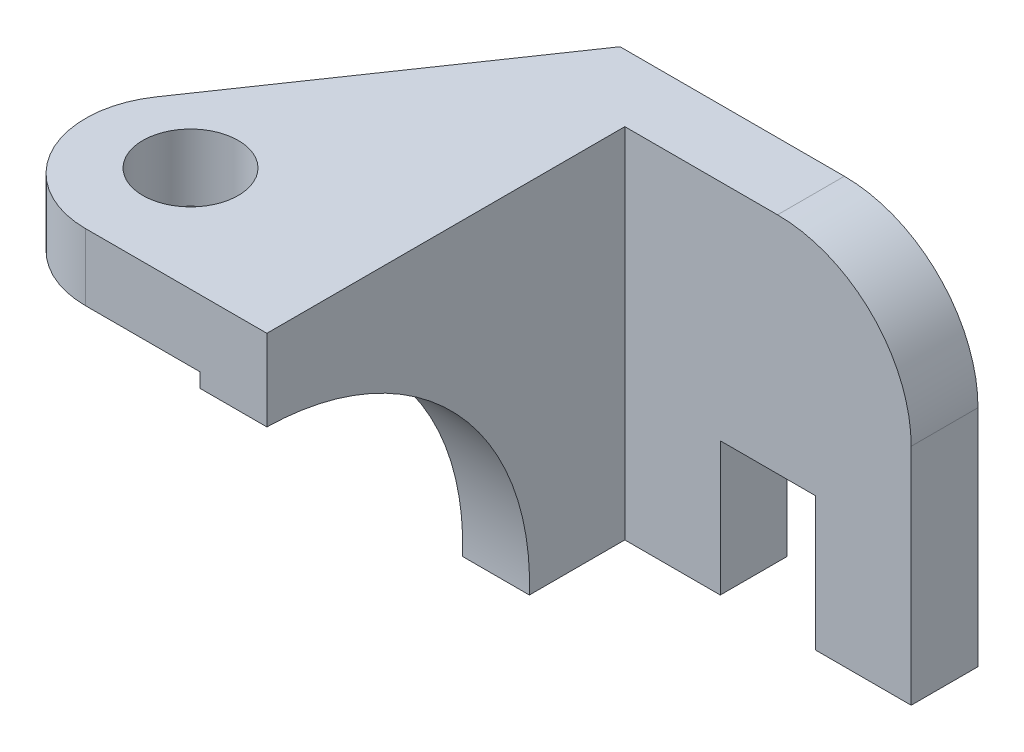
ISO-10303-21;
HEADER;
FILE_DESCRIPTION(('STEP AP214'),'2;1');
FILE_NAME('part.step','',(''),(''),'','','');
FILE_SCHEMA(('AUTOMOTIVE_DESIGN { 1 0 10303 214 1 1 1 1 }'));
ENDSEC;
DATA;
#1=APPLICATION_CONTEXT('core data for automotive mechanical design processes');
#2=APPLICATION_PROTOCOL_DEFINITION('international standard','automotive_design',2000,#1);
#3=PRODUCT_CONTEXT('',#1,'mechanical');
#4=PRODUCT('Part','Part','',(#3));
#5=PRODUCT_RELATED_PRODUCT_CATEGORY('part','',(#4));
#6=PRODUCT_DEFINITION_FORMATION('','',#4);
#7=PRODUCT_DEFINITION_CONTEXT('part definition',#1,'design');
#8=PRODUCT_DEFINITION('design','',#6,#7);
#9=PRODUCT_DEFINITION_SHAPE('','',#8);
#10=(LENGTH_UNIT() NAMED_UNIT(*) SI_UNIT(.MILLI.,.METRE.));
#11=(NAMED_UNIT(*) PLANE_ANGLE_UNIT() SI_UNIT($,.RADIAN.));
#12=(NAMED_UNIT(*) SI_UNIT($,.STERADIAN.) SOLID_ANGLE_UNIT());
#13=UNCERTAINTY_MEASURE_WITH_UNIT(LENGTH_MEASURE(1.E-05),#10,'distance_accuracy_value','');
#14=(GEOMETRIC_REPRESENTATION_CONTEXT(3) GLOBAL_UNCERTAINTY_ASSIGNED_CONTEXT((#13)) GLOBAL_UNIT_ASSIGNED_CONTEXT((#10,
#11,#12)) REPRESENTATION_CONTEXT('',''));
#15=CARTESIAN_POINT('',(0.,0.,0.));
#16=DIRECTION('',(0.,0.,1.));
#17=DIRECTION('',(1.,0.,0.));
#18=AXIS2_PLACEMENT_3D('',#15,#16,#17);
#19=CARTESIAN_POINT('',(0.,0.,14.));
#20=DIRECTION('',(0.,0.,-1.));
#21=DIRECTION('',(-1.,0.,0.));
#22=AXIS2_PLACEMENT_3D('',#19,#20,#21);
#23=PLANE('',#22);
#24=DIRECTION('',(0.,1.,0.));
#25=VECTOR('',#24,1.);
#26=CARTESIAN_POINT('',(75.,75.,14.));
#27=LINE('',#26,#25);
#28=CARTESIAN_POINT('',(75.,0.,14.));
#29=VERTEX_POINT('',#28);
#30=CARTESIAN_POINT('',(75.,47.,14.));
#31=VERTEX_POINT('',#30);
#32=EDGE_CURVE('E223',#29,#31,#27,.T.);
#33=ORIENTED_EDGE('',*,*,#32,.T.);
#34=CARTESIAN_POINT('',(47.,47.,14.));
#35=DIRECTION('',(0.,0.,-1.));
#36=DIRECTION('',(-1.,0.,0.));
#37=AXIS2_PLACEMENT_3D('',#34,#35,#36);
#38=CIRCLE('',#37,28.);
#39=CARTESIAN_POINT('',(47.,75.,14.));
#40=VERTEX_POINT('',#39);
#41=EDGE_CURVE('E11',#31,#40,#38,.F.);
#42=ORIENTED_EDGE('',*,*,#41,.T.);
#43=DIRECTION('',(-1.,0.,0.));
#44=VECTOR('',#43,1.);
#45=CARTESIAN_POINT('',(1.,75.,14.));
#46=LINE('',#45,#44);
#47=CARTESIAN_POINT('',(15.,75.,14.));
#48=VERTEX_POINT('',#47);
#49=EDGE_CURVE('E230',#40,#48,#46,.T.);
#50=ORIENTED_EDGE('',*,*,#49,.T.);
#51=DIRECTION('',(0.,1.,0.));
#52=VECTOR('',#51,1.);
#53=CARTESIAN_POINT('',(15.,75.,14.));
#54=LINE('',#53,#52);
#55=CARTESIAN_POINT('',(15.,0.,14.));
#56=VERTEX_POINT('',#55);
#57=EDGE_CURVE('E186',#56,#48,#54,.T.);
#58=ORIENTED_EDGE('',*,*,#57,.F.);
#59=DIRECTION('',(1.,0.,0.));
#60=VECTOR('',#59,1.);
#61=CARTESIAN_POINT('',(35.,0.,14.));
#62=LINE('',#61,#60);
#63=CARTESIAN_POINT('',(35.,0.,14.));
#64=VERTEX_POINT('',#63);
#65=EDGE_CURVE('E214',#56,#64,#62,.T.);
#66=ORIENTED_EDGE('',*,*,#65,.T.);
#67=DIRECTION('',(0.,1.,0.));
#68=VECTOR('',#67,1.);
#69=CARTESIAN_POINT('',(35.,28.,14.));
#70=LINE('',#69,#68);
#71=CARTESIAN_POINT('',(35.,28.,14.));
#72=VERTEX_POINT('',#71);
#73=EDGE_CURVE('E220',#64,#72,#70,.T.);
#74=ORIENTED_EDGE('',*,*,#73,.T.);
#75=DIRECTION('',(1.,0.,0.));
#76=VECTOR('',#75,1.);
#77=CARTESIAN_POINT('',(55.,28.,14.));
#78=LINE('',#77,#76);
#79=CARTESIAN_POINT('',(55.,28.,14.));
#80=VERTEX_POINT('',#79);
#81=EDGE_CURVE('E218',#72,#80,#78,.T.);
#82=ORIENTED_EDGE('',*,*,#81,.T.);
#83=DIRECTION('',(0.,-1.,0.));
#84=VECTOR('',#83,1.);
#85=CARTESIAN_POINT('',(55.,0.,14.));
#86=LINE('',#85,#84);
#87=CARTESIAN_POINT('',(55.,0.,14.));
#88=VERTEX_POINT('',#87);
#89=EDGE_CURVE('E222',#80,#88,#86,.T.);
#90=ORIENTED_EDGE('',*,*,#89,.T.);
#91=DIRECTION('',(1.,0.,0.));
#92=VECTOR('',#91,1.);
#93=CARTESIAN_POINT('',(75.,0.,14.));
#94=LINE('',#93,#92);
#95=EDGE_CURVE('E224',#88,#29,#94,.T.);
#96=ORIENTED_EDGE('',*,*,#95,.T.);
#97=EDGE_LOOP('',(#33,#42,#50,#58,#66,#74,#82,#90,#96));
#98=FACE_BOUND('',#97,.T.);
#99=ADVANCED_FACE('F39',(#98),#23,.F.);
#100=CARTESIAN_POINT('',(35.,0.,14.));
#101=DIRECTION('',(0.,1.,0.));
#102=DIRECTION('',(-1.,0.,0.));
#103=AXIS2_PLACEMENT_3D('',#100,#101,#102);
#104=PLANE('',#103);
#105=DIRECTION('',(1.,0.,0.));
#106=VECTOR('',#105,1.);
#107=CARTESIAN_POINT('',(35.,0.,0.));
#108=LINE('',#107,#106);
#109=CARTESIAN_POINT('',(1.,0.,0.));
#110=VERTEX_POINT('',#109);
#111=CARTESIAN_POINT('',(35.,0.,0.));
#112=VERTEX_POINT('',#111);
#113=EDGE_CURVE('E212',#110,#112,#108,.T.);
#114=ORIENTED_EDGE('',*,*,#113,.T.);
#115=DIRECTION('',(0.,0.,-1.));
#116=VECTOR('',#115,1.);
#117=CARTESIAN_POINT('',(35.,0.,14.));
#118=LINE('',#117,#116);
#119=EDGE_CURVE('E259',#64,#112,#118,.T.);
#120=ORIENTED_EDGE('',*,*,#119,.F.);
#121=ORIENTED_EDGE('',*,*,#65,.F.);
#122=DIRECTION('',(0.,0.,-1.));
#123=VECTOR('',#122,1.);
#124=CARTESIAN_POINT('',(15.,0.,14.));
#125=LINE('',#124,#123);
#126=CARTESIAN_POINT('',(15.,0.,34.));
#127=VERTEX_POINT('',#126);
#128=EDGE_CURVE('E199',#127,#56,#125,.T.);
#129=ORIENTED_EDGE('',*,*,#128,.F.);
#130=DIRECTION('',(-1.,0.,0.));
#131=VECTOR('',#130,1.);
#132=CARTESIAN_POINT('',(15.,0.,34.));
#133=LINE('',#132,#131);
#134=CARTESIAN_POINT('',(1.,0.,34.));
#135=VERTEX_POINT('',#134);
#136=EDGE_CURVE('E201',#127,#135,#133,.T.);
#137=ORIENTED_EDGE('',*,*,#136,.T.);
#138=DIRECTION('',(0.,0.,-1.));
#139=VECTOR('',#138,1.);
#140=CARTESIAN_POINT('',(1.,0.,14.));
#141=LINE('',#140,#139);
#142=EDGE_CURVE('E229',#135,#110,#141,.T.);
#143=ORIENTED_EDGE('',*,*,#142,.T.);
#144=EDGE_LOOP('',(#114,#120,#121,#129,#137,#143));
#145=FACE_BOUND('',#144,.T.);
#146=ADVANCED_FACE('F300',(#145),#104,.F.);
#147=CARTESIAN_POINT('',(35.,28.,14.));
#148=DIRECTION('',(-1.,0.,0.));
#149=DIRECTION('',(0.,0.,1.));
#150=AXIS2_PLACEMENT_3D('',#147,#148,#149);
#151=PLANE('',#150);
#152=DIRECTION('',(0.,1.,0.));
#153=VECTOR('',#152,1.);
#154=CARTESIAN_POINT('',(35.,28.,0.));
#155=LINE('',#154,#153);
#156=CARTESIAN_POINT('',(35.,28.,0.));
#157=VERTEX_POINT('',#156);
#158=EDGE_CURVE('E235',#112,#157,#155,.T.);
#159=ORIENTED_EDGE('',*,*,#158,.T.);
#160=DIRECTION('',(0.,0.,-1.));
#161=VECTOR('',#160,1.);
#162=CARTESIAN_POINT('',(35.,28.,14.));
#163=LINE('',#162,#161);
#164=EDGE_CURVE('E258',#72,#157,#163,.T.);
#165=ORIENTED_EDGE('',*,*,#164,.F.);
#166=ORIENTED_EDGE('',*,*,#73,.F.);
#167=ORIENTED_EDGE('',*,*,#119,.T.);
#168=EDGE_LOOP('',(#159,#165,#166,#167));
#169=FACE_BOUND('',#168,.T.);
#170=ADVANCED_FACE('F294',(#169),#151,.F.);
#171=CARTESIAN_POINT('',(55.,28.,14.));
#172=DIRECTION('',(0.,1.,0.));
#173=DIRECTION('',(-1.,0.,0.));
#174=AXIS2_PLACEMENT_3D('',#171,#172,#173);
#175=PLANE('',#174);
#176=DIRECTION('',(1.,0.,0.));
#177=VECTOR('',#176,1.);
#178=CARTESIAN_POINT('',(55.,28.,0.));
#179=LINE('',#178,#177);
#180=CARTESIAN_POINT('',(55.,28.,0.));
#181=VERTEX_POINT('',#180);
#182=EDGE_CURVE('E231',#157,#181,#179,.T.);
#183=ORIENTED_EDGE('',*,*,#182,.T.);
#184=DIRECTION('',(0.,0.,-1.));
#185=VECTOR('',#184,1.);
#186=CARTESIAN_POINT('',(55.,28.,14.));
#187=LINE('',#186,#185);
#188=EDGE_CURVE('E251',#80,#181,#187,.T.);
#189=ORIENTED_EDGE('',*,*,#188,.F.);
#190=ORIENTED_EDGE('',*,*,#81,.F.);
#191=ORIENTED_EDGE('',*,*,#164,.T.);
#192=EDGE_LOOP('',(#183,#189,#190,#191));
#193=FACE_BOUND('',#192,.T.);
#194=ADVANCED_FACE('F286',(#193),#175,.F.);
#195=CARTESIAN_POINT('',(55.,0.,14.));
#196=DIRECTION('',(1.,0.,0.));
#197=DIRECTION('',(0.,1.,0.));
#198=AXIS2_PLACEMENT_3D('',#195,#196,#197);
#199=PLANE('',#198);
#200=DIRECTION('',(0.,-1.,0.));
#201=VECTOR('',#200,1.);
#202=CARTESIAN_POINT('',(55.,0.,0.));
#203=LINE('',#202,#201);
#204=CARTESIAN_POINT('',(55.,0.,0.));
#205=VERTEX_POINT('',#204);
#206=EDGE_CURVE('E237',#181,#205,#203,.T.);
#207=ORIENTED_EDGE('',*,*,#206,.T.);
#208=DIRECTION('',(0.,0.,-1.));
#209=VECTOR('',#208,1.);
#210=CARTESIAN_POINT('',(55.,0.,14.));
#211=LINE('',#210,#209);
#212=EDGE_CURVE('E248',#88,#205,#211,.T.);
#213=ORIENTED_EDGE('',*,*,#212,.F.);
#214=ORIENTED_EDGE('',*,*,#89,.F.);
#215=ORIENTED_EDGE('',*,*,#188,.T.);
#216=EDGE_LOOP('',(#207,#213,#214,#215));
#217=FACE_BOUND('',#216,.T.);
#218=ADVANCED_FACE('F281',(#217),#199,.F.);
#219=CARTESIAN_POINT('',(75.,0.,14.));
#220=DIRECTION('',(0.,1.,0.));
#221=DIRECTION('',(-1.,0.,0.));
#222=AXIS2_PLACEMENT_3D('',#219,#220,#221);
#223=PLANE('',#222);
#224=DIRECTION('',(1.,0.,0.));
#225=VECTOR('',#224,1.);
#226=CARTESIAN_POINT('',(75.,0.,0.));
#227=LINE('',#226,#225);
#228=CARTESIAN_POINT('',(75.,0.,0.));
#229=VERTEX_POINT('',#228);
#230=EDGE_CURVE('E236',#205,#229,#227,.T.);
#231=ORIENTED_EDGE('',*,*,#230,.T.);
#232=DIRECTION('',(0.,0.,-1.));
#233=VECTOR('',#232,1.);
#234=CARTESIAN_POINT('',(75.,0.,14.));
#235=LINE('',#234,#233);
#236=EDGE_CURVE('E250',#29,#229,#235,.T.);
#237=ORIENTED_EDGE('',*,*,#236,.F.);
#238=ORIENTED_EDGE('',*,*,#95,.F.);
#239=ORIENTED_EDGE('',*,*,#212,.T.);
#240=EDGE_LOOP('',(#231,#237,#238,#239));
#241=FACE_BOUND('',#240,.T.);
#242=ADVANCED_FACE('F282',(#241),#223,.F.);
#243=CARTESIAN_POINT('',(75.,75.,14.));
#244=DIRECTION('',(-1.,0.,0.));
#245=DIRECTION('',(0.,-1.,0.));
#246=AXIS2_PLACEMENT_3D('',#243,#244,#245);
#247=PLANE('',#246);
#248=DIRECTION('',(0.,1.,0.));
#249=VECTOR('',#248,1.);
#250=CARTESIAN_POINT('',(75.,75.,0.));
#251=LINE('',#250,#249);
#252=CARTESIAN_POINT('',(75.,47.,0.));
#253=VERTEX_POINT('',#252);
#254=EDGE_CURVE('E238',#229,#253,#251,.T.);
#255=ORIENTED_EDGE('',*,*,#254,.T.);
#256=DIRECTION('',(0.,0.,-1.));
#257=VECTOR('',#256,1.);
#258=CARTESIAN_POINT('',(75.,47.,14.));
#259=LINE('',#258,#257);
#260=EDGE_CURVE('E50',#253,#31,#259,.F.);
#261=ORIENTED_EDGE('',*,*,#260,.T.);
#262=ORIENTED_EDGE('',*,*,#32,.F.);
#263=ORIENTED_EDGE('',*,*,#236,.T.);
#264=EDGE_LOOP('',(#255,#261,#262,#263));
#265=FACE_BOUND('',#264,.T.);
#266=ADVANCED_FACE('F277',(#265),#247,.F.);
#267=CARTESIAN_POINT('',(1.,75.,14.));
#268=DIRECTION('',(0.,-1.,0.));
#269=DIRECTION('',(1.,0.,0.));
#270=AXIS2_PLACEMENT_3D('',#267,#268,#269);
#271=PLANE('',#270);
#272=ORIENTED_EDGE('',*,*,#49,.F.);
#273=DIRECTION('',(0.,0.,-1.));
#274=VECTOR('',#273,1.);
#275=CARTESIAN_POINT('',(47.,75.,14.));
#276=LINE('',#275,#274);
#277=CARTESIAN_POINT('',(47.,75.,0.));
#278=VERTEX_POINT('',#277);
#279=EDGE_CURVE('E265',#40,#278,#276,.T.);
#280=ORIENTED_EDGE('',*,*,#279,.T.);
#281=DIRECTION('',(-1.,0.,0.));
#282=VECTOR('',#281,1.);
#283=CARTESIAN_POINT('',(1.,75.,0.));
#284=LINE('',#283,#282);
#285=CARTESIAN_POINT('',(0.,75.,0.));
#286=VERTEX_POINT('',#285);
#287=EDGE_CURVE('E245',#278,#286,#284,.T.);
#288=ORIENTED_EDGE('',*,*,#287,.T.);
#289=DIRECTION('',(-0.564906673687776,0.,0.825154803672022));
#290=VECTOR('',#289,1.);
#291=CARTESIAN_POINT('',(-39.5030960734404,75.,57.7018665262445));
#292=LINE('',#291,#290);
#293=CARTESIAN_POINT('',(-39.5030960734404,75.,57.7018665262445));
#294=VERTEX_POINT('',#293);
#295=EDGE_CURVE('E155',#286,#294,#292,.T.);
#296=ORIENTED_EDGE('',*,*,#295,.T.);
#297=CARTESIAN_POINT('',(-23.,75.,69.));
#298=DIRECTION('',(0.,1.,0.));
#299=DIRECTION('',(-1.,0.,0.));
#300=AXIS2_PLACEMENT_3D('',#297,#298,#299);
#301=CIRCLE('',#300,20.);
#302=CARTESIAN_POINT('',(-23.,75.,89.));
#303=VERTEX_POINT('',#302);
#304=EDGE_CURVE('E172',#294,#303,#301,.T.);
#305=ORIENTED_EDGE('',*,*,#304,.T.);
#306=DIRECTION('',(-1.,0.,0.));
#307=VECTOR('',#306,1.);
#308=CARTESIAN_POINT('',(15.,75.,89.));
#309=LINE('',#308,#307);
#310=CARTESIAN_POINT('',(15.,75.,89.));
#311=VERTEX_POINT('',#310);
#312=EDGE_CURVE('E215',#311,#303,#309,.T.);
#313=ORIENTED_EDGE('',*,*,#312,.F.);
#314=DIRECTION('',(0.,0.,1.));
#315=VECTOR('',#314,1.);
#316=CARTESIAN_POINT('',(15.,75.,14.));
#317=LINE('',#316,#315);
#318=EDGE_CURVE('E194',#48,#311,#317,.T.);
#319=ORIENTED_EDGE('',*,*,#318,.F.);
#320=EDGE_LOOP('',(#272,#280,#288,#296,#305,#313,#319));
#321=FACE_BOUND('',#320,.T.);
#322=CARTESIAN_POINT('',(-23.,75.,67.));
#323=DIRECTION('',(0.,1.,0.));
#324=DIRECTION('',(-1.,0.,0.));
#325=AXIS2_PLACEMENT_3D('',#322,#323,#324);
#326=CIRCLE('',#325,10.);
#327=CARTESIAN_POINT('',(-33.,75.,67.));
#328=VERTEX_POINT('',#327);
#329=EDGE_CURVE('E177',#328,#328,#326,.T.);
#330=ORIENTED_EDGE('',*,*,#329,.F.);
#331=EDGE_LOOP('',(#330));
#332=FACE_BOUND('',#331,.T.);
#333=ADVANCED_FACE('F268',(#321,#332),#271,.F.);
#334=CARTESIAN_POINT('',(1.,0.,14.));
#335=DIRECTION('',(1.,0.,0.));
#336=DIRECTION('',(0.,0.,-1.));
#337=AXIS2_PLACEMENT_3D('',#334,#335,#336);
#338=PLANE('',#337);
#339=DIRECTION('',(0.,-1.,0.));
#340=VECTOR('',#339,1.);
#341=CARTESIAN_POINT('',(1.,75.,89.));
#342=LINE('',#341,#340);
#343=CARTESIAN_POINT('',(0.999999999999997,61.,89.));
#344=VERTEX_POINT('',#343);
#345=CARTESIAN_POINT('',(1.,58.,89.));
#346=VERTEX_POINT('',#345);
#347=EDGE_CURVE('E188',#344,#346,#342,.T.);
#348=ORIENTED_EDGE('',*,*,#347,.F.);
#349=DIRECTION('',(0.,0.,-1.));
#350=VECTOR('',#349,1.);
#351=CARTESIAN_POINT('',(0.999999999999997,61.,0.));
#352=LINE('',#351,#350);
#353=CARTESIAN_POINT('',(1.,61.,0.));
#354=VERTEX_POINT('',#353);
#355=EDGE_CURVE('E154',#344,#354,#352,.T.);
#356=ORIENTED_EDGE('',*,*,#355,.T.);
#357=DIRECTION('',(0.,-1.,0.));
#358=VECTOR('',#357,1.);
#359=CARTESIAN_POINT('',(1.,0.,0.));
#360=LINE('',#359,#358);
#361=EDGE_CURVE('E168',#354,#110,#360,.T.);
#362=ORIENTED_EDGE('',*,*,#361,.T.);
#363=ORIENTED_EDGE('',*,*,#142,.F.);
#364=CARTESIAN_POINT('',(1.,2.00829750750392,89.963977173905));
#365=DIRECTION('',(-1.,0.,0.));
#366=DIRECTION('',(0.,0.,1.));
#367=AXIS2_PLACEMENT_3D('',#364,#365,#366);
#368=CIRCLE('',#367,56.);
#369=EDGE_CURVE('E191',#346,#135,#368,.T.);
#370=ORIENTED_EDGE('',*,*,#369,.F.);
#371=EDGE_LOOP('',(#348,#356,#362,#363,#370));
#372=FACE_BOUND('',#371,.T.);
#373=ADVANCED_FACE('F304',(#372),#338,.F.);
#374=CARTESIAN_POINT('',(0.,0.,0.));
#375=DIRECTION('',(0.,0.,-1.));
#376=DIRECTION('',(-1.,0.,0.));
#377=AXIS2_PLACEMENT_3D('',#374,#375,#376);
#378=PLANE('',#377);
#379=ORIENTED_EDGE('',*,*,#287,.F.);
#380=CARTESIAN_POINT('',(47.,47.,0.));
#381=DIRECTION('',(0.,0.,-1.));
#382=DIRECTION('',(-1.,0.,0.));
#383=AXIS2_PLACEMENT_3D('',#380,#381,#382);
#384=CIRCLE('',#383,28.);
#385=EDGE_CURVE('E62',#278,#253,#384,.T.);
#386=ORIENTED_EDGE('',*,*,#385,.T.);
#387=ORIENTED_EDGE('',*,*,#254,.F.);
#388=ORIENTED_EDGE('',*,*,#230,.F.);
#389=ORIENTED_EDGE('',*,*,#206,.F.);
#390=ORIENTED_EDGE('',*,*,#182,.F.);
#391=ORIENTED_EDGE('',*,*,#158,.F.);
#392=ORIENTED_EDGE('',*,*,#113,.F.);
#393=ORIENTED_EDGE('',*,*,#361,.F.);
#394=DIRECTION('',(-1.,0.,0.));
#395=VECTOR('',#394,1.);
#396=CARTESIAN_POINT('',(0.,61.,0.));
#397=LINE('',#396,#395);
#398=CARTESIAN_POINT('',(0.,61.,0.));
#399=VERTEX_POINT('',#398);
#400=EDGE_CURVE('E161',#354,#399,#397,.T.);
#401=ORIENTED_EDGE('',*,*,#400,.T.);
#402=DIRECTION('',(0.,1.,0.));
#403=VECTOR('',#402,1.);
#404=CARTESIAN_POINT('',(0.,61.,0.));
#405=LINE('',#404,#403);
#406=EDGE_CURVE('E150',#399,#286,#405,.T.);
#407=ORIENTED_EDGE('',*,*,#406,.T.);
#408=EDGE_LOOP('',(#379,#386,#387,#388,#389,#390,#391,#392,#393,#401,#407));
#409=FACE_BOUND('',#408,.T.);
#410=ADVANCED_FACE('F169',(#409),#378,.T.);
#411=CARTESIAN_POINT('',(15.,75.,89.));
#412=DIRECTION('',(0.,0.,-1.));
#413=DIRECTION('',(-1.,0.,0.));
#414=AXIS2_PLACEMENT_3D('',#411,#412,#413);
#415=PLANE('',#414);
#416=ORIENTED_EDGE('',*,*,#312,.T.);
#417=DIRECTION('',(0.,1.,0.));
#418=VECTOR('',#417,1.);
#419=CARTESIAN_POINT('',(-23.,61.,89.));
#420=LINE('',#419,#418);
#421=CARTESIAN_POINT('',(-23.,61.,89.));
#422=VERTEX_POINT('',#421);
#423=EDGE_CURVE('E183',#422,#303,#420,.T.);
#424=ORIENTED_EDGE('',*,*,#423,.F.);
#425=DIRECTION('',(1.,0.,0.));
#426=VECTOR('',#425,1.);
#427=CARTESIAN_POINT('',(0.999999999999997,61.,89.));
#428=LINE('',#427,#426);
#429=EDGE_CURVE('E178',#422,#344,#428,.T.);
#430=ORIENTED_EDGE('',*,*,#429,.T.);
#431=ORIENTED_EDGE('',*,*,#347,.T.);
#432=DIRECTION('',(-1.,0.,0.));
#433=VECTOR('',#432,1.);
#434=CARTESIAN_POINT('',(15.,58.,89.));
#435=LINE('',#434,#433);
#436=CARTESIAN_POINT('',(15.,58.,89.));
#437=VERTEX_POINT('',#436);
#438=EDGE_CURVE('E207',#437,#346,#435,.T.);
#439=ORIENTED_EDGE('',*,*,#438,.F.);
#440=DIRECTION('',(0.,-1.,0.));
#441=VECTOR('',#440,1.);
#442=CARTESIAN_POINT('',(15.,75.,89.));
#443=LINE('',#442,#441);
#444=EDGE_CURVE('E198',#311,#437,#443,.T.);
#445=ORIENTED_EDGE('',*,*,#444,.F.);
#446=EDGE_LOOP('',(#416,#424,#430,#431,#439,#445));
#447=FACE_BOUND('',#446,.T.);
#448=ADVANCED_FACE('F309',(#447),#415,.F.);
#449=CARTESIAN_POINT('',(15.,2.00829750750392,89.963977173905));
#450=DIRECTION('',(-1.,0.,0.));
#451=DIRECTION('',(0.,0.,1.));
#452=AXIS2_PLACEMENT_3D('',#449,#450,#451);
#453=CYLINDRICAL_SURFACE('',#452,56.);
#454=ORIENTED_EDGE('',*,*,#369,.T.);
#455=ORIENTED_EDGE('',*,*,#136,.F.);
#456=CARTESIAN_POINT('',(15.,2.00829750750392,89.963977173905));
#457=DIRECTION('',(-1.,0.,0.));
#458=DIRECTION('',(0.,0.,1.));
#459=AXIS2_PLACEMENT_3D('',#456,#457,#458);
#460=CIRCLE('',#459,56.);
#461=EDGE_CURVE('E196',#437,#127,#460,.T.);
#462=ORIENTED_EDGE('',*,*,#461,.F.);
#463=ORIENTED_EDGE('',*,*,#438,.T.);
#464=EDGE_LOOP('',(#454,#455,#462,#463));
#465=FACE_BOUND('',#464,.T.);
#466=ADVANCED_FACE('F303',(#465),#453,.F.);
#467=CARTESIAN_POINT('',(15.,2.00829750750392,89.963977173905));
#468=DIRECTION('',(-1.,0.,0.));
#469=DIRECTION('',(0.,0.,1.));
#470=AXIS2_PLACEMENT_3D('',#467,#468,#469);
#471=PLANE('',#470);
#472=ORIENTED_EDGE('',*,*,#57,.T.);
#473=ORIENTED_EDGE('',*,*,#318,.T.);
#474=ORIENTED_EDGE('',*,*,#444,.T.);
#475=ORIENTED_EDGE('',*,*,#461,.T.);
#476=ORIENTED_EDGE('',*,*,#128,.T.);
#477=EDGE_LOOP('',(#472,#473,#474,#475,#476));
#478=FACE_BOUND('',#477,.T.);
#479=ADVANCED_FACE('F316',(#478),#471,.F.);
#480=CARTESIAN_POINT('',(-23.,61.,69.));
#481=DIRECTION('',(0.,1.,0.));
#482=DIRECTION('',(-1.,0.,0.));
#483=AXIS2_PLACEMENT_3D('',#480,#481,#482);
#484=CYLINDRICAL_SURFACE('',#483,20.);
#485=ORIENTED_EDGE('',*,*,#304,.F.);
#486=DIRECTION('',(0.,1.,0.));
#487=VECTOR('',#486,1.);
#488=CARTESIAN_POINT('',(-39.5030960734404,61.,57.7018665262445));
#489=LINE('',#488,#487);
#490=CARTESIAN_POINT('',(-39.5030960734404,61.,57.7018665262445));
#491=VERTEX_POINT('',#490);
#492=EDGE_CURVE('E152',#491,#294,#489,.T.);
#493=ORIENTED_EDGE('',*,*,#492,.F.);
#494=CARTESIAN_POINT('',(-23.,61.,69.));
#495=DIRECTION('',(0.,1.,0.));
#496=DIRECTION('',(-1.,0.,0.));
#497=AXIS2_PLACEMENT_3D('',#494,#495,#496);
#498=CIRCLE('',#497,20.);
#499=EDGE_CURVE('E164',#491,#422,#498,.T.);
#500=ORIENTED_EDGE('',*,*,#499,.T.);
#501=ORIENTED_EDGE('',*,*,#423,.T.);
#502=EDGE_LOOP('',(#485,#493,#500,#501));
#503=FACE_BOUND('',#502,.T.);
#504=ADVANCED_FACE('F311',(#503),#484,.T.);
#505=CARTESIAN_POINT('',(-39.5030960734404,61.,57.7018665262445));
#506=DIRECTION('',(-0.825154803672022,0.,-0.564906673687776));
#507=DIRECTION('',(-0.564906673687776,0.,0.825154803672022));
#508=AXIS2_PLACEMENT_3D('',#505,#506,#507);
#509=PLANE('',#508);
#510=ORIENTED_EDGE('',*,*,#295,.F.);
#511=ORIENTED_EDGE('',*,*,#406,.F.);
#512=DIRECTION('',(-0.564906673687776,0.,0.825154803672022));
#513=VECTOR('',#512,1.);
#514=CARTESIAN_POINT('',(-39.5030960734404,61.,57.7018665262445));
#515=LINE('',#514,#513);
#516=EDGE_CURVE('E147',#399,#491,#515,.T.);
#517=ORIENTED_EDGE('',*,*,#516,.T.);
#518=ORIENTED_EDGE('',*,*,#492,.T.);
#519=EDGE_LOOP('',(#510,#511,#517,#518));
#520=FACE_BOUND('',#519,.T.);
#521=ADVANCED_FACE('F149',(#520),#509,.T.);
#522=CARTESIAN_POINT('',(-23.,61.,69.));
#523=DIRECTION('',(0.,1.,0.));
#524=DIRECTION('',(-1.,0.,0.));
#525=AXIS2_PLACEMENT_3D('',#522,#523,#524);
#526=PLANE('',#525);
#527=CARTESIAN_POINT('',(-23.,61.,67.));
#528=DIRECTION('',(0.,1.,0.));
#529=DIRECTION('',(-1.,0.,0.));
#530=AXIS2_PLACEMENT_3D('',#527,#528,#529);
#531=CIRCLE('',#530,10.);
#532=CARTESIAN_POINT('',(-33.,61.,67.));
#533=VERTEX_POINT('',#532);
#534=EDGE_CURVE('E181',#533,#533,#531,.T.);
#535=ORIENTED_EDGE('',*,*,#534,.T.);
#536=EDGE_LOOP('',(#535));
#537=FACE_BOUND('',#536,.T.);
#538=ORIENTED_EDGE('',*,*,#400,.F.);
#539=ORIENTED_EDGE('',*,*,#355,.F.);
#540=ORIENTED_EDGE('',*,*,#429,.F.);
#541=ORIENTED_EDGE('',*,*,#499,.F.);
#542=ORIENTED_EDGE('',*,*,#516,.F.);
#543=EDGE_LOOP('',(#538,#539,#540,#541,#542));
#544=FACE_BOUND('',#543,.T.);
#545=ADVANCED_FACE('F157',(#537,#544),#526,.F.);
#546=CARTESIAN_POINT('',(-23.,61.,67.));
#547=DIRECTION('',(0.,1.,0.));
#548=DIRECTION('',(-1.,0.,0.));
#549=AXIS2_PLACEMENT_3D('',#546,#547,#548);
#550=CYLINDRICAL_SURFACE('',#549,10.);
#551=ORIENTED_EDGE('',*,*,#534,.F.);
#552=EDGE_LOOP('',(#551));
#553=FACE_BOUND('',#552,.T.);
#554=ORIENTED_EDGE('',*,*,#329,.T.);
#555=EDGE_LOOP('',(#554));
#556=FACE_BOUND('',#555,.T.);
#557=ADVANCED_FACE('F433',(#553,#556),#550,.F.);
#558=CARTESIAN_POINT('',(47.,47.,14.));
#559=DIRECTION('',(0.,0.,-1.));
#560=DIRECTION('',(-1.,0.,0.));
#561=AXIS2_PLACEMENT_3D('',#558,#559,#560);
#562=CYLINDRICAL_SURFACE('',#561,28.);
#563=ORIENTED_EDGE('',*,*,#41,.F.);
#564=ORIENTED_EDGE('',*,*,#260,.F.);
#565=ORIENTED_EDGE('',*,*,#385,.F.);
#566=ORIENTED_EDGE('',*,*,#279,.F.);
#567=EDGE_LOOP('',(#563,#564,#565,#566));
#568=FACE_BOUND('',#567,.T.);
#569=ADVANCED_FACE('F41',(#568),#562,.T.);
#570=CLOSED_SHELL('',(#99,#146,#170,#194,#218,#242,#266,#333,#373,#410,#448,#466,#479,#504,#521,
#545,#557,#569));
#571=MANIFOLD_SOLID_BREP('B2',#570);
#572=ADVANCED_BREP_SHAPE_REPRESENTATION('',(#18,#571),#14);
#573=SHAPE_DEFINITION_REPRESENTATION(#9,#572);
ENDSEC;
END-ISO-10303-21;
